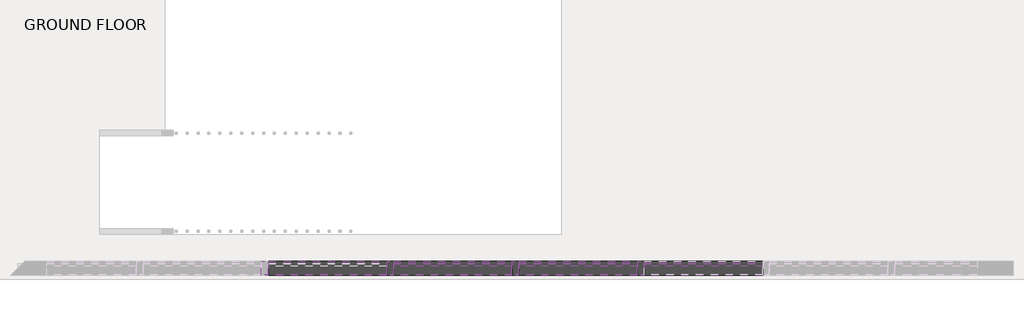
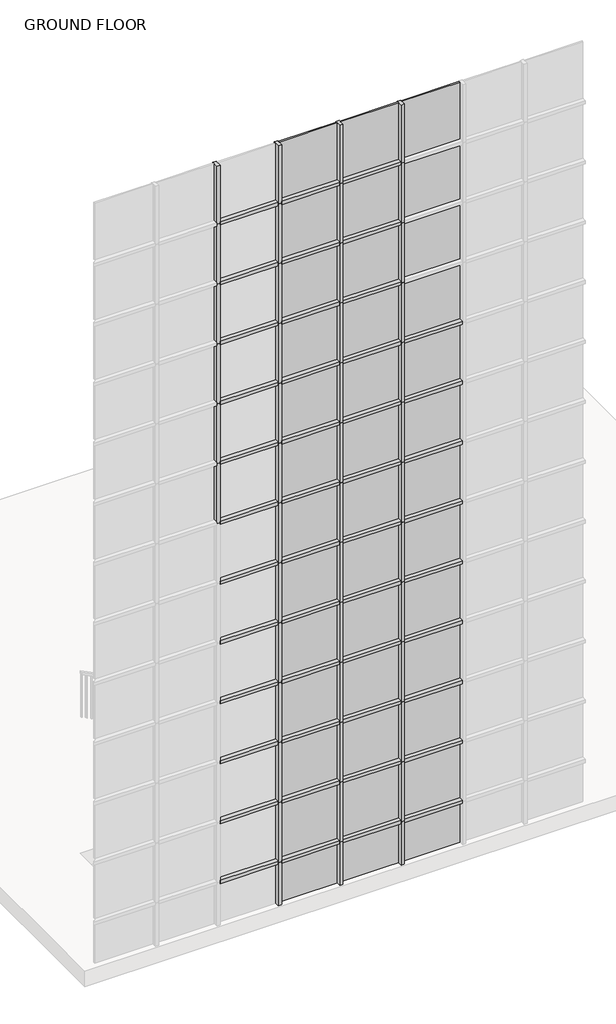
# One storey, part 3 of 16: 90 members, 39 plates.
"""IFC4 building model written with IfcOpenShell, lengths in millimetres."""

from ifc_helpers import new_model, si_unit, origin, place, context, project, spatial, transform, mapped, element, save
from components import member_d518c94e, member_b860638c, member_31fee25f, system_panel_glazed_5cba32e5

model = new_model("IFC4")

# Units and contexts
model_context = context("Model", 3, world=origin())
ifc_project = project(units=[si_unit("LENGTHUNIT", "METRE", prefix="MILLI")], contexts=[model_context])

# Site, building, storey
site = spatial("IfcSite", under=ifc_project)
building = spatial("IfcBuilding", under=site)
storey = spatial("IfcBuildingStorey", under=building, Name="GROUND FLOOR", Elevation=0.0)

# Members
placement = place(None, origin())
member_shape = member_d518c94e(model_context)
element("IfcMember", 1, ObjectType="Rectangular Mullion : 2.5\" x 5\" rectangular", at=placement, inside=storey, context=model_context, shape_type="MappedRepresentation", body=[
    mapped(member_shape, transform((-5691.994061, -5739.2238032, 1168.8884615), x_axis=(0.0, 0.0, 1.0), y_axis=(0.0, -1.0, 0.0), z_axis=(1.0, 0.0, 0.0))),
])
element("IfcMember", 2, ObjectType="Rectangular Mullion : 2.5\" x 5\" rectangular", at=placement, inside=storey, context=model_context, shape_type="MappedRepresentation", body=[
    mapped(member_shape, transform((-4526.5248302, -5739.2238032, 1168.8884615), x_axis=(0.0, 0.0, 1.0), y_axis=(0.0, -1.0, 0.0), z_axis=(1.0, 0.0, 0.0))),
])
element("IfcMember", 3, ObjectType="Rectangular Mullion : 2.5\" x 5\" rectangular", at=placement, inside=storey, context=model_context, shape_type="MappedRepresentation", body=[
    mapped(member_shape, transform((-3361.0555995, -5739.2238032, 1168.8884615), x_axis=(0.0, 0.0, 1.0), y_axis=(0.0, -1.0, 0.0), z_axis=(1.0, 0.0, 0.0))),
])
element("IfcMember", 4, ObjectType="Rectangular Mullion : 2.5\" x 5\" rectangular", at=placement, inside=storey, context=model_context, shape_type="MappedRepresentation", body=[
    mapped(member_shape, transform((-2195.5863688, -5739.2238032, 1168.8884615), x_axis=(0.0, 0.0, 1.0), y_axis=(0.0, -1.0, 0.0), z_axis=(1.0, 0.0, 0.0))),
])
element("IfcMember", 5, ObjectType="Rectangular Mullion : 2.5\" x 5\" rectangular", at=placement, inside=storey, context=model_context, shape_type="MappedRepresentation", body=[
    mapped(member_shape, transform((-5691.994061, -5739.2238032, 2369.5269231), x_axis=(0.0, 0.0, 1.0), y_axis=(0.0, -1.0, 0.0), z_axis=(1.0, 0.0, 0.0))),
])
element("IfcMember", 6, ObjectType="Rectangular Mullion : 2.5\" x 5\" rectangular", at=placement, inside=storey, context=model_context, shape_type="MappedRepresentation", body=[
    mapped(member_shape, transform((-4526.5248302, -5739.2238032, 2369.5269231), x_axis=(0.0, 0.0, 1.0), y_axis=(0.0, -1.0, 0.0), z_axis=(1.0, 0.0, 0.0))),
])
element("IfcMember", 7, ObjectType="Rectangular Mullion : 2.5\" x 5\" rectangular", at=placement, inside=storey, context=model_context, shape_type="MappedRepresentation", body=[
    mapped(member_shape, transform((-3361.0555995, -5739.2238032, 2369.5269231), x_axis=(0.0, 0.0, 1.0), y_axis=(0.0, -1.0, 0.0), z_axis=(1.0, 0.0, 0.0))),
])
element("IfcMember", 8, ObjectType="Rectangular Mullion : 2.5\" x 5\" rectangular", at=placement, inside=storey, context=model_context, shape_type="MappedRepresentation", body=[
    mapped(member_shape, transform((-2195.5863688, -5739.2238032, 2369.5269231), x_axis=(0.0, 0.0, 1.0), y_axis=(0.0, -1.0, 0.0), z_axis=(1.0, 0.0, 0.0))),
])
element("IfcMember", 9, ObjectType="Rectangular Mullion : 2.5\" x 5\" rectangular", at=placement, inside=storey, context=model_context, shape_type="MappedRepresentation", body=[
    mapped(member_shape, transform((-5691.994061, -5739.2238032, 3570.1653846), x_axis=(0.0, 0.0, 1.0), y_axis=(0.0, -1.0, 0.0), z_axis=(1.0, 0.0, 0.0))),
])
element("IfcMember", 10, ObjectType="Rectangular Mullion : 2.5\" x 5\" rectangular", at=placement, inside=storey, context=model_context, shape_type="MappedRepresentation", body=[
    mapped(member_shape, transform((-4526.5248302, -5739.2238032, 3570.1653846), x_axis=(0.0, 0.0, 1.0), y_axis=(0.0, -1.0, 0.0), z_axis=(1.0, 0.0, 0.0))),
])
element("IfcMember", 11, ObjectType="Rectangular Mullion : 2.5\" x 5\" rectangular", at=placement, inside=storey, context=model_context, shape_type="MappedRepresentation", body=[
    mapped(member_shape, transform((-3361.0555995, -5739.2238032, 3570.1653846), x_axis=(0.0, 0.0, 1.0), y_axis=(0.0, -1.0, 0.0), z_axis=(1.0, 0.0, 0.0))),
])
element("IfcMember", 12, ObjectType="Rectangular Mullion : 2.5\" x 5\" rectangular", at=placement, inside=storey, context=model_context, shape_type="MappedRepresentation", body=[
    mapped(member_shape, transform((-2195.5863688, -5739.2238032, 3570.1653846), x_axis=(0.0, 0.0, 1.0), y_axis=(0.0, -1.0, 0.0), z_axis=(1.0, 0.0, 0.0))),
])
element("IfcMember", 13, ObjectType="Rectangular Mullion : 2.5\" x 5\" rectangular", at=placement, inside=storey, context=model_context, shape_type="MappedRepresentation", body=[
    mapped(member_shape, transform((-5691.994061, -5739.2238032, 4770.8038462), x_axis=(0.0, 0.0, 1.0), y_axis=(0.0, -1.0, 0.0), z_axis=(1.0, 0.0, 0.0))),
])
element("IfcMember", 14, ObjectType="Rectangular Mullion : 2.5\" x 5\" rectangular", at=placement, inside=storey, context=model_context, shape_type="MappedRepresentation", body=[
    mapped(member_shape, transform((-4526.5248302, -5739.2238032, 4770.8038462), x_axis=(0.0, 0.0, 1.0), y_axis=(0.0, -1.0, 0.0), z_axis=(1.0, 0.0, 0.0))),
])
element("IfcMember", 15, ObjectType="Rectangular Mullion : 2.5\" x 5\" rectangular", at=placement, inside=storey, context=model_context, shape_type="MappedRepresentation", body=[
    mapped(member_shape, transform((-3361.0555995, -5739.2238032, 4770.8038462), x_axis=(0.0, 0.0, 1.0), y_axis=(0.0, -1.0, 0.0), z_axis=(1.0, 0.0, 0.0))),
])
element("IfcMember", 16, ObjectType="Rectangular Mullion : 2.5\" x 5\" rectangular", at=placement, inside=storey, context=model_context, shape_type="MappedRepresentation", body=[
    mapped(member_shape, transform((-2195.5863688, -5739.2238032, 4770.8038462), x_axis=(0.0, 0.0, 1.0), y_axis=(0.0, -1.0, 0.0), z_axis=(1.0, 0.0, 0.0))),
])
element("IfcMember", 17, ObjectType="Rectangular Mullion : 2.5\" x 5\" rectangular", at=placement, inside=storey, context=model_context, shape_type="MappedRepresentation", body=[
    mapped(member_shape, transform((-5691.994061, -5739.2238032, 5971.4423077), x_axis=(0.0, 0.0, 1.0), y_axis=(0.0, -1.0, 0.0), z_axis=(1.0, 0.0, 0.0))),
])
element("IfcMember", 18, ObjectType="Rectangular Mullion : 2.5\" x 5\" rectangular", at=placement, inside=storey, context=model_context, shape_type="MappedRepresentation", body=[
    mapped(member_shape, transform((-4526.5248302, -5739.2238032, 5971.4423077), x_axis=(0.0, 0.0, 1.0), y_axis=(0.0, -1.0, 0.0), z_axis=(1.0, 0.0, 0.0))),
])
element("IfcMember", 19, ObjectType="Rectangular Mullion : 2.5\" x 5\" rectangular", at=placement, inside=storey, context=model_context, shape_type="MappedRepresentation", body=[
    mapped(member_shape, transform((-3361.0555995, -5739.2238032, 5971.4423077), x_axis=(0.0, 0.0, 1.0), y_axis=(0.0, -1.0, 0.0), z_axis=(1.0, 0.0, 0.0))),
])
element("IfcMember", 20, ObjectType="Rectangular Mullion : 2.5\" x 5\" rectangular", at=placement, inside=storey, context=model_context, shape_type="MappedRepresentation", body=[
    mapped(member_shape, transform((-2195.5863688, -5739.2238032, 5971.4423077), x_axis=(0.0, 0.0, 1.0), y_axis=(0.0, -1.0, 0.0), z_axis=(1.0, 0.0, 0.0))),
])
element("IfcMember", 21, ObjectType="Rectangular Mullion : 2.5\" x 5\" rectangular", at=placement, inside=storey, context=model_context, shape_type="MappedRepresentation", body=[
    mapped(member_shape, transform((-5691.994061, -5739.2238032, 7172.0807692), x_axis=(0.0, 0.0, 1.0), y_axis=(0.0, -1.0, 0.0), z_axis=(1.0, 0.0, 0.0))),
])
element("IfcMember", 22, ObjectType="Rectangular Mullion : 2.5\" x 5\" rectangular", at=placement, inside=storey, context=model_context, shape_type="MappedRepresentation", body=[
    mapped(member_shape, transform((-4526.5248302, -5739.2238032, 7172.0807692), x_axis=(0.0, 0.0, 1.0), y_axis=(0.0, -1.0, 0.0), z_axis=(1.0, 0.0, 0.0))),
])
element("IfcMember", 23, ObjectType="Rectangular Mullion : 2.5\" x 5\" rectangular", at=placement, inside=storey, context=model_context, shape_type="MappedRepresentation", body=[
    mapped(member_shape, transform((-3361.0555995, -5739.2238032, 7172.0807692), x_axis=(0.0, 0.0, 1.0), y_axis=(0.0, -1.0, 0.0), z_axis=(1.0, 0.0, 0.0))),
])
element("IfcMember", 24, ObjectType="Rectangular Mullion : 2.5\" x 5\" rectangular", at=placement, inside=storey, context=model_context, shape_type="MappedRepresentation", body=[
    mapped(member_shape, transform((-2195.5863688, -5739.2238032, 7172.0807692), x_axis=(0.0, 0.0, 1.0), y_axis=(0.0, -1.0, 0.0), z_axis=(1.0, 0.0, 0.0))),
])
element("IfcMember", 25, ObjectType="Rectangular Mullion : 2.5\" x 5\" rectangular", at=placement, inside=storey, context=model_context, shape_type="MappedRepresentation", body=[
    mapped(member_shape, transform((-5691.994061, -5739.2238032, 8372.7192308), x_axis=(0.0, 0.0, 1.0), y_axis=(0.0, -1.0, 0.0), z_axis=(1.0, 0.0, 0.0))),
])
element("IfcMember", 26, ObjectType="Rectangular Mullion : 2.5\" x 5\" rectangular", at=placement, inside=storey, context=model_context, shape_type="MappedRepresentation", body=[
    mapped(member_shape, transform((-4526.5248302, -5739.2238032, 8372.7192308), x_axis=(0.0, 0.0, 1.0), y_axis=(0.0, -1.0, 0.0), z_axis=(1.0, 0.0, 0.0))),
])
element("IfcMember", 27, ObjectType="Rectangular Mullion : 2.5\" x 5\" rectangular", at=placement, inside=storey, context=model_context, shape_type="MappedRepresentation", body=[
    mapped(member_shape, transform((-3361.0555995, -5739.2238032, 8372.7192308), x_axis=(0.0, 0.0, 1.0), y_axis=(0.0, -1.0, 0.0), z_axis=(1.0, 0.0, 0.0))),
])
element("IfcMember", 28, ObjectType="Rectangular Mullion : 2.5\" x 5\" rectangular", at=placement, inside=storey, context=model_context, shape_type="MappedRepresentation", body=[
    mapped(member_shape, transform((-2195.5863688, -5739.2238032, 8372.7192308), x_axis=(0.0, 0.0, 1.0), y_axis=(0.0, -1.0, 0.0), z_axis=(1.0, 0.0, 0.0))),
])
element("IfcMember", 29, ObjectType="Rectangular Mullion : 2.5\" x 5\" rectangular", at=placement, inside=storey, context=model_context, shape_type="MappedRepresentation", body=[
    mapped(member_shape, transform((-5691.994061, -5739.2238032, 9573.3576923), x_axis=(0.0, 0.0, 1.0), y_axis=(0.0, -1.0, 0.0), z_axis=(1.0, 0.0, 0.0))),
])
element("IfcMember", 30, ObjectType="Rectangular Mullion : 2.5\" x 5\" rectangular", at=placement, inside=storey, context=model_context, shape_type="MappedRepresentation", body=[
    mapped(member_shape, transform((-4526.5248302, -5739.2238032, 9573.3576923), x_axis=(0.0, 0.0, 1.0), y_axis=(0.0, -1.0, 0.0), z_axis=(1.0, 0.0, 0.0))),
])
element("IfcMember", 31, ObjectType="Rectangular Mullion : 2.5\" x 5\" rectangular", at=placement, inside=storey, context=model_context, shape_type="MappedRepresentation", body=[
    mapped(member_shape, transform((-3361.0555995, -5739.2238032, 9573.3576923), x_axis=(0.0, 0.0, 1.0), y_axis=(0.0, -1.0, 0.0), z_axis=(1.0, 0.0, 0.0))),
])
element("IfcMember", 32, ObjectType="Rectangular Mullion : 2.5\" x 5\" rectangular", at=placement, inside=storey, context=model_context, shape_type="MappedRepresentation", body=[
    mapped(member_shape, transform((-2195.5863688, -5739.2238032, 9573.3576923), x_axis=(0.0, 0.0, 1.0), y_axis=(0.0, -1.0, 0.0), z_axis=(1.0, 0.0, 0.0))),
])
element("IfcMember", 33, ObjectType="Rectangular Mullion : 2.5\" x 5\" rectangular", at=placement, inside=storey, context=model_context, shape_type="MappedRepresentation", body=[
    mapped(member_shape, transform((-5691.994061, -5739.2238032, 10773.9961538), x_axis=(0.0, 0.0, 1.0), y_axis=(0.0, -1.0, 0.0), z_axis=(1.0, 0.0, 0.0))),
])
element("IfcMember", 34, ObjectType="Rectangular Mullion : 2.5\" x 5\" rectangular", at=placement, inside=storey, context=model_context, shape_type="MappedRepresentation", body=[
    mapped(member_shape, transform((-4526.5248302, -5739.2238032, 10773.9961538), x_axis=(0.0, 0.0, 1.0), y_axis=(0.0, -1.0, 0.0), z_axis=(1.0, 0.0, 0.0))),
])
element("IfcMember", 35, ObjectType="Rectangular Mullion : 2.5\" x 5\" rectangular", at=placement, inside=storey, context=model_context, shape_type="MappedRepresentation", body=[
    mapped(member_shape, transform((-3361.0555995, -5739.2238032, 10773.9961538), x_axis=(0.0, 0.0, 1.0), y_axis=(0.0, -1.0, 0.0), z_axis=(1.0, 0.0, 0.0))),
])
element("IfcMember", 36, ObjectType="Rectangular Mullion : 2.5\" x 5\" rectangular", at=placement, inside=storey, context=model_context, shape_type="MappedRepresentation", body=[
    mapped(member_shape, transform((-2195.5863688, -5739.2238032, 10773.9961538), x_axis=(0.0, 0.0, 1.0), y_axis=(0.0, -1.0, 0.0), z_axis=(1.0, 0.0, 0.0))),
])
element("IfcMember", 37, ObjectType="Rectangular Mullion : 2.5\" x 5\" rectangular", at=placement, inside=storey, context=model_context, shape_type="MappedRepresentation", body=[
    mapped(member_shape, transform((-5691.994061, -5739.2238032, 11974.6346154), x_axis=(0.0, 0.0, 1.0), y_axis=(0.0, -1.0, 0.0), z_axis=(1.0, 0.0, 0.0))),
])
element("IfcMember", 38, ObjectType="Rectangular Mullion : 2.5\" x 5\" rectangular", at=placement, inside=storey, context=model_context, shape_type="MappedRepresentation", body=[
    mapped(member_shape, transform((-4526.5248302, -5739.2238032, 11974.6346154), x_axis=(0.0, 0.0, 1.0), y_axis=(0.0, -1.0, 0.0), z_axis=(1.0, 0.0, 0.0))),
])
element("IfcMember", 39, ObjectType="Rectangular Mullion : 2.5\" x 5\" rectangular", at=placement, inside=storey, context=model_context, shape_type="MappedRepresentation", body=[
    mapped(member_shape, transform((-3361.0555995, -5739.2238032, 11974.6346154), x_axis=(0.0, 0.0, 1.0), y_axis=(0.0, -1.0, 0.0), z_axis=(1.0, 0.0, 0.0))),
])
element("IfcMember", 40, ObjectType="Rectangular Mullion : 2.5\" x 5\" rectangular", at=placement, inside=storey, context=model_context, shape_type="MappedRepresentation", body=[
    mapped(member_shape, transform((-5691.994061, -5739.2238032, 13175.2730769), x_axis=(0.0, 0.0, 1.0), y_axis=(0.0, -1.0, 0.0), z_axis=(1.0, 0.0, 0.0))),
])
element("IfcMember", 41, ObjectType="Rectangular Mullion : 2.5\" x 5\" rectangular", at=placement, inside=storey, context=model_context, shape_type="MappedRepresentation", body=[
    mapped(member_shape, transform((-4526.5248302, -5739.2238032, 13175.2730769), x_axis=(0.0, 0.0, 1.0), y_axis=(0.0, -1.0, 0.0), z_axis=(1.0, 0.0, 0.0))),
])
element("IfcMember", 42, ObjectType="Rectangular Mullion : 2.5\" x 5\" rectangular", at=placement, inside=storey, context=model_context, shape_type="MappedRepresentation", body=[
    mapped(member_shape, transform((-3361.0555995, -5739.2238032, 13175.2730769), x_axis=(0.0, 0.0, 1.0), y_axis=(0.0, -1.0, 0.0), z_axis=(1.0, 0.0, 0.0))),
])
element("IfcMember", 43, ObjectType="Rectangular Mullion : 2.5\" x 5\" rectangular", at=placement, inside=storey, context=model_context, shape_type="MappedRepresentation", body=[
    mapped(member_shape, transform((-5691.994061, -5739.2238032, 14375.9115385), x_axis=(0.0, 0.0, 1.0), y_axis=(0.0, -1.0, 0.0), z_axis=(1.0, 0.0, 0.0))),
])
element("IfcMember", 44, ObjectType="Rectangular Mullion : 2.5\" x 5\" rectangular", at=placement, inside=storey, context=model_context, shape_type="MappedRepresentation", body=[
    mapped(member_shape, transform((-4526.5248302, -5739.2238032, 14375.9115385), x_axis=(0.0, 0.0, 1.0), y_axis=(0.0, -1.0, 0.0), z_axis=(1.0, 0.0, 0.0))),
])
element("IfcMember", 45, ObjectType="Rectangular Mullion : 2.5\" x 5\" rectangular", at=placement, inside=storey, context=model_context, shape_type="MappedRepresentation", body=[
    mapped(member_shape, transform((-3361.0555995, -5739.2238032, 14375.9115385), x_axis=(0.0, 0.0, 1.0), y_axis=(0.0, -1.0, 0.0), z_axis=(1.0, 0.0, 0.0))),
])
member_2_shape = member_b860638c(model_context)
element("IfcMember", 46, ObjectType="Rectangular Mullion : 2.5\" x 5\" rectangular", at=placement, inside=storey, context=model_context, shape_type="MappedRepresentation", body=[
    mapped(member_2_shape, transform((-5660.244061, -5739.2238032, 0.0), x_axis=(1.0, 0.0, 0.0), y_axis=(0.0, -1.0, 0.0), z_axis=(0.0, 0.0, -1.0))),
])
element("IfcMember", 47, ObjectType="Rectangular Mullion : 2.5\" x 5\" rectangular", at=placement, inside=storey, context=model_context, shape_type="MappedRepresentation", body=[
    mapped(member_2_shape, transform((-4494.7748302, -5739.2238032, 0.0), x_axis=(1.0, 0.0, 0.0), y_axis=(0.0, -1.0, 0.0), z_axis=(0.0, 0.0, -1.0))),
])
element("IfcMember", 48, ObjectType="Rectangular Mullion : 2.5\" x 5\" rectangular", at=placement, inside=storey, context=model_context, shape_type="MappedRepresentation", body=[
    mapped(member_2_shape, transform((-3329.3055995, -5739.2238032, 0.0), x_axis=(1.0, 0.0, 0.0), y_axis=(0.0, -1.0, 0.0), z_axis=(0.0, 0.0, -1.0))),
])
member_3_shape = member_31fee25f(model_context)
element("IfcMember", 49, ObjectType="Rectangular Mullion : 2.5\" x 5\" rectangular", at=placement, inside=storey, context=model_context, shape_type="MappedRepresentation", body=[
    mapped(member_3_shape, transform((-5660.244061, -5739.2238032, 1168.8884615), x_axis=(1.0, 0.0, 0.0), y_axis=(0.0, -1.0, 0.0), z_axis=(0.0, 0.0, -1.0))),
])
element("IfcMember", 50, ObjectType="Rectangular Mullion : 2.5\" x 5\" rectangular", at=placement, inside=storey, context=model_context, shape_type="MappedRepresentation", body=[
    mapped(member_3_shape, transform((-4494.7748302, -5739.2238032, 1168.8884615), x_axis=(1.0, 0.0, 0.0), y_axis=(0.0, -1.0, 0.0), z_axis=(0.0, 0.0, -1.0))),
])
element("IfcMember", 51, ObjectType="Rectangular Mullion : 2.5\" x 5\" rectangular", at=placement, inside=storey, context=model_context, shape_type="MappedRepresentation", body=[
    mapped(member_3_shape, transform((-3329.3055995, -5739.2238032, 1168.8884615), x_axis=(1.0, 0.0, 0.0), y_axis=(0.0, -1.0, 0.0), z_axis=(0.0, 0.0, -1.0))),
])
element("IfcMember", 52, ObjectType="Rectangular Mullion : 2.5\" x 5\" rectangular", at=placement, inside=storey, context=model_context, shape_type="MappedRepresentation", body=[
    mapped(member_3_shape, transform((-5660.244061, -5739.2238032, 2369.5269231), x_axis=(1.0, 0.0, 0.0), y_axis=(0.0, -1.0, 0.0), z_axis=(0.0, 0.0, -1.0))),
])
element("IfcMember", 53, ObjectType="Rectangular Mullion : 2.5\" x 5\" rectangular", at=placement, inside=storey, context=model_context, shape_type="MappedRepresentation", body=[
    mapped(member_3_shape, transform((-4494.7748302, -5739.2238032, 2369.5269231), x_axis=(1.0, 0.0, 0.0), y_axis=(0.0, -1.0, 0.0), z_axis=(0.0, 0.0, -1.0))),
])
element("IfcMember", 54, ObjectType="Rectangular Mullion : 2.5\" x 5\" rectangular", at=placement, inside=storey, context=model_context, shape_type="MappedRepresentation", body=[
    mapped(member_3_shape, transform((-3329.3055995, -5739.2238032, 2369.5269231), x_axis=(1.0, 0.0, 0.0), y_axis=(0.0, -1.0, 0.0), z_axis=(0.0, 0.0, -1.0))),
])
element("IfcMember", 55, ObjectType="Rectangular Mullion : 2.5\" x 5\" rectangular", at=placement, inside=storey, context=model_context, shape_type="MappedRepresentation", body=[
    mapped(member_3_shape, transform((-5660.244061, -5739.2238032, 3570.1653846), x_axis=(1.0, 0.0, 0.0), y_axis=(0.0, -1.0, 0.0), z_axis=(0.0, 0.0, -1.0))),
])
element("IfcMember", 56, ObjectType="Rectangular Mullion : 2.5\" x 5\" rectangular", at=placement, inside=storey, context=model_context, shape_type="MappedRepresentation", body=[
    mapped(member_3_shape, transform((-4494.7748302, -5739.2238032, 3570.1653846), x_axis=(1.0, 0.0, 0.0), y_axis=(0.0, -1.0, 0.0), z_axis=(0.0, 0.0, -1.0))),
])
element("IfcMember", 57, ObjectType="Rectangular Mullion : 2.5\" x 5\" rectangular", at=placement, inside=storey, context=model_context, shape_type="MappedRepresentation", body=[
    mapped(member_3_shape, transform((-3329.3055995, -5739.2238032, 3570.1653846), x_axis=(1.0, 0.0, 0.0), y_axis=(0.0, -1.0, 0.0), z_axis=(0.0, 0.0, -1.0))),
])
element("IfcMember", 58, ObjectType="Rectangular Mullion : 2.5\" x 5\" rectangular", at=placement, inside=storey, context=model_context, shape_type="MappedRepresentation", body=[
    mapped(member_3_shape, transform((-5660.244061, -5739.2238032, 4770.8038462), x_axis=(1.0, 0.0, 0.0), y_axis=(0.0, -1.0, 0.0), z_axis=(0.0, 0.0, -1.0))),
])
element("IfcMember", 59, ObjectType="Rectangular Mullion : 2.5\" x 5\" rectangular", at=placement, inside=storey, context=model_context, shape_type="MappedRepresentation", body=[
    mapped(member_3_shape, transform((-4494.7748302, -5739.2238032, 4770.8038462), x_axis=(1.0, 0.0, 0.0), y_axis=(0.0, -1.0, 0.0), z_axis=(0.0, 0.0, -1.0))),
])
element("IfcMember", 60, ObjectType="Rectangular Mullion : 2.5\" x 5\" rectangular", at=placement, inside=storey, context=model_context, shape_type="MappedRepresentation", body=[
    mapped(member_3_shape, transform((-3329.3055995, -5739.2238032, 4770.8038462), x_axis=(1.0, 0.0, 0.0), y_axis=(0.0, -1.0, 0.0), z_axis=(0.0, 0.0, -1.0))),
])
element("IfcMember", 61, ObjectType="Rectangular Mullion : 2.5\" x 5\" rectangular", at=placement, inside=storey, context=model_context, shape_type="MappedRepresentation", body=[
    mapped(member_3_shape, transform((-5660.244061, -5739.2238032, 5971.4423077), x_axis=(1.0, 0.0, 0.0), y_axis=(0.0, -1.0, 0.0), z_axis=(0.0, 0.0, -1.0))),
])
element("IfcMember", 62, ObjectType="Rectangular Mullion : 2.5\" x 5\" rectangular", at=placement, inside=storey, context=model_context, shape_type="MappedRepresentation", body=[
    mapped(member_3_shape, transform((-4494.7748302, -5739.2238032, 5971.4423077), x_axis=(1.0, 0.0, 0.0), y_axis=(0.0, -1.0, 0.0), z_axis=(0.0, 0.0, -1.0))),
])
element("IfcMember", 63, ObjectType="Rectangular Mullion : 2.5\" x 5\" rectangular", at=placement, inside=storey, context=model_context, shape_type="MappedRepresentation", body=[
    mapped(member_3_shape, transform((-3329.3055995, -5739.2238032, 5971.4423077), x_axis=(1.0, 0.0, 0.0), y_axis=(0.0, -1.0, 0.0), z_axis=(0.0, 0.0, -1.0))),
])
element("IfcMember", 64, ObjectType="Rectangular Mullion : 2.5\" x 5\" rectangular", at=placement, inside=storey, context=model_context, shape_type="MappedRepresentation", body=[
    mapped(member_3_shape, transform((-5660.244061, -5739.2238032, 7172.0807692), x_axis=(1.0, 0.0, 0.0), y_axis=(0.0, -1.0, 0.0), z_axis=(0.0, 0.0, -1.0))),
])
element("IfcMember", 65, ObjectType="Rectangular Mullion : 2.5\" x 5\" rectangular", at=placement, inside=storey, context=model_context, shape_type="MappedRepresentation", body=[
    mapped(member_3_shape, transform((-4494.7748302, -5739.2238032, 7172.0807692), x_axis=(1.0, 0.0, 0.0), y_axis=(0.0, -1.0, 0.0), z_axis=(0.0, 0.0, -1.0))),
])
element("IfcMember", 66, ObjectType="Rectangular Mullion : 2.5\" x 5\" rectangular", at=placement, inside=storey, context=model_context, shape_type="MappedRepresentation", body=[
    mapped(member_3_shape, transform((-3329.3055995, -5739.2238032, 7172.0807692), x_axis=(1.0, 0.0, 0.0), y_axis=(0.0, -1.0, 0.0), z_axis=(0.0, 0.0, -1.0))),
])
element("IfcMember", 67, ObjectType="Rectangular Mullion : 2.5\" x 5\" rectangular", at=placement, inside=storey, context=model_context, shape_type="MappedRepresentation", body=[
    mapped(member_3_shape, transform((-6825.7132917, -5739.2238032, 8372.7192308), x_axis=(1.0, 0.0, 0.0), y_axis=(0.0, -1.0, 0.0), z_axis=(0.0, 0.0, -1.0))),
])
element("IfcMember", 68, ObjectType="Rectangular Mullion : 2.5\" x 5\" rectangular", at=placement, inside=storey, context=model_context, shape_type="MappedRepresentation", body=[
    mapped(member_3_shape, transform((-5660.244061, -5739.2238032, 8372.7192308), x_axis=(1.0, 0.0, 0.0), y_axis=(0.0, -1.0, 0.0), z_axis=(0.0, 0.0, -1.0))),
])
element("IfcMember", 69, ObjectType="Rectangular Mullion : 2.5\" x 5\" rectangular", at=placement, inside=storey, context=model_context, shape_type="MappedRepresentation", body=[
    mapped(member_3_shape, transform((-4494.7748302, -5739.2238032, 8372.7192308), x_axis=(1.0, 0.0, 0.0), y_axis=(0.0, -1.0, 0.0), z_axis=(0.0, 0.0, -1.0))),
])
element("IfcMember", 70, ObjectType="Rectangular Mullion : 2.5\" x 5\" rectangular", at=placement, inside=storey, context=model_context, shape_type="MappedRepresentation", body=[
    mapped(member_3_shape, transform((-3329.3055995, -5739.2238032, 8372.7192308), x_axis=(1.0, 0.0, 0.0), y_axis=(0.0, -1.0, 0.0), z_axis=(0.0, 0.0, -1.0))),
])
element("IfcMember", 71, ObjectType="Rectangular Mullion : 2.5\" x 5\" rectangular", at=placement, inside=storey, context=model_context, shape_type="MappedRepresentation", body=[
    mapped(member_3_shape, transform((-6825.7132917, -5739.2238032, 9573.3576923), x_axis=(1.0, 0.0, 0.0), y_axis=(0.0, -1.0, 0.0), z_axis=(0.0, 0.0, -1.0))),
])
element("IfcMember", 72, ObjectType="Rectangular Mullion : 2.5\" x 5\" rectangular", at=placement, inside=storey, context=model_context, shape_type="MappedRepresentation", body=[
    mapped(member_3_shape, transform((-5660.244061, -5739.2238032, 9573.3576923), x_axis=(1.0, 0.0, 0.0), y_axis=(0.0, -1.0, 0.0), z_axis=(0.0, 0.0, -1.0))),
])
element("IfcMember", 73, ObjectType="Rectangular Mullion : 2.5\" x 5\" rectangular", at=placement, inside=storey, context=model_context, shape_type="MappedRepresentation", body=[
    mapped(member_3_shape, transform((-4494.7748302, -5739.2238032, 9573.3576923), x_axis=(1.0, 0.0, 0.0), y_axis=(0.0, -1.0, 0.0), z_axis=(0.0, 0.0, -1.0))),
])
element("IfcMember", 74, ObjectType="Rectangular Mullion : 2.5\" x 5\" rectangular", at=placement, inside=storey, context=model_context, shape_type="MappedRepresentation", body=[
    mapped(member_3_shape, transform((-3329.3055995, -5739.2238032, 9573.3576923), x_axis=(1.0, 0.0, 0.0), y_axis=(0.0, -1.0, 0.0), z_axis=(0.0, 0.0, -1.0))),
])
element("IfcMember", 75, ObjectType="Rectangular Mullion : 2.5\" x 5\" rectangular", at=placement, inside=storey, context=model_context, shape_type="MappedRepresentation", body=[
    mapped(member_3_shape, transform((-6825.7132917, -5739.2238032, 10773.9961538), x_axis=(1.0, 0.0, 0.0), y_axis=(0.0, -1.0, 0.0), z_axis=(0.0, 0.0, -1.0))),
])
element("IfcMember", 76, ObjectType="Rectangular Mullion : 2.5\" x 5\" rectangular", at=placement, inside=storey, context=model_context, shape_type="MappedRepresentation", body=[
    mapped(member_3_shape, transform((-5660.244061, -5739.2238032, 10773.9961538), x_axis=(1.0, 0.0, 0.0), y_axis=(0.0, -1.0, 0.0), z_axis=(0.0, 0.0, -1.0))),
])
element("IfcMember", 77, ObjectType="Rectangular Mullion : 2.5\" x 5\" rectangular", at=placement, inside=storey, context=model_context, shape_type="MappedRepresentation", body=[
    mapped(member_3_shape, transform((-4494.7748302, -5739.2238032, 10773.9961538), x_axis=(1.0, 0.0, 0.0), y_axis=(0.0, -1.0, 0.0), z_axis=(0.0, 0.0, -1.0))),
])
element("IfcMember", 78, ObjectType="Rectangular Mullion : 2.5\" x 5\" rectangular", at=placement, inside=storey, context=model_context, shape_type="MappedRepresentation", body=[
    mapped(member_3_shape, transform((-3329.3055995, -5739.2238032, 10773.9961538), x_axis=(1.0, 0.0, 0.0), y_axis=(0.0, -1.0, 0.0), z_axis=(0.0, 0.0, -1.0))),
])
element("IfcMember", 79, ObjectType="Rectangular Mullion : 2.5\" x 5\" rectangular", at=placement, inside=storey, context=model_context, shape_type="MappedRepresentation", body=[
    mapped(member_3_shape, transform((-6825.7132917, -5739.2238032, 11974.6346154), x_axis=(1.0, 0.0, 0.0), y_axis=(0.0, -1.0, 0.0), z_axis=(0.0, 0.0, -1.0))),
])
element("IfcMember", 80, ObjectType="Rectangular Mullion : 2.5\" x 5\" rectangular", at=placement, inside=storey, context=model_context, shape_type="MappedRepresentation", body=[
    mapped(member_3_shape, transform((-5660.244061, -5739.2238032, 11974.6346154), x_axis=(1.0, 0.0, 0.0), y_axis=(0.0, -1.0, 0.0), z_axis=(0.0, 0.0, -1.0))),
])
element("IfcMember", 81, ObjectType="Rectangular Mullion : 2.5\" x 5\" rectangular", at=placement, inside=storey, context=model_context, shape_type="MappedRepresentation", body=[
    mapped(member_3_shape, transform((-4494.7748302, -5739.2238032, 11974.6346154), x_axis=(1.0, 0.0, 0.0), y_axis=(0.0, -1.0, 0.0), z_axis=(0.0, 0.0, -1.0))),
])
element("IfcMember", 82, ObjectType="Rectangular Mullion : 2.5\" x 5\" rectangular", at=placement, inside=storey, context=model_context, shape_type="MappedRepresentation", body=[
    mapped(member_3_shape, transform((-3329.3055995, -5739.2238032, 11974.6346154), x_axis=(1.0, 0.0, 0.0), y_axis=(0.0, -1.0, 0.0), z_axis=(0.0, 0.0, -1.0))),
])
element("IfcMember", 83, ObjectType="Rectangular Mullion : 2.5\" x 5\" rectangular", at=placement, inside=storey, context=model_context, shape_type="MappedRepresentation", body=[
    mapped(member_3_shape, transform((-6825.7132917, -5739.2238032, 13175.2730769), x_axis=(1.0, 0.0, 0.0), y_axis=(0.0, -1.0, 0.0), z_axis=(0.0, 0.0, -1.0))),
])
element("IfcMember", 84, ObjectType="Rectangular Mullion : 2.5\" x 5\" rectangular", at=placement, inside=storey, context=model_context, shape_type="MappedRepresentation", body=[
    mapped(member_3_shape, transform((-5660.244061, -5739.2238032, 13175.2730769), x_axis=(1.0, 0.0, 0.0), y_axis=(0.0, -1.0, 0.0), z_axis=(0.0, 0.0, -1.0))),
])
element("IfcMember", 85, ObjectType="Rectangular Mullion : 2.5\" x 5\" rectangular", at=placement, inside=storey, context=model_context, shape_type="MappedRepresentation", body=[
    mapped(member_3_shape, transform((-4494.7748302, -5739.2238032, 13175.2730769), x_axis=(1.0, 0.0, 0.0), y_axis=(0.0, -1.0, 0.0), z_axis=(0.0, 0.0, -1.0))),
])
element("IfcMember", 86, ObjectType="Rectangular Mullion : 2.5\" x 5\" rectangular", at=placement, inside=storey, context=model_context, shape_type="MappedRepresentation", body=[
    mapped(member_3_shape, transform((-3329.3055995, -5739.2238032, 13175.2730769), x_axis=(1.0, 0.0, 0.0), y_axis=(0.0, -1.0, 0.0), z_axis=(0.0, 0.0, -1.0))),
])
element("IfcMember", 87, ObjectType="Rectangular Mullion : 2.5\" x 5\" rectangular", at=placement, inside=storey, context=model_context, shape_type="MappedRepresentation", body=[
    mapped(member_2_shape, transform((-6825.7132917, -5739.2238032, 14375.9115385), x_axis=(1.0, 0.0, 0.0), y_axis=(0.0, -1.0, 0.0), z_axis=(0.0, 0.0, -1.0))),
])
element("IfcMember", 88, ObjectType="Rectangular Mullion : 2.5\" x 5\" rectangular", at=placement, inside=storey, context=model_context, shape_type="MappedRepresentation", body=[
    mapped(member_2_shape, transform((-5660.244061, -5739.2238032, 14375.9115385), x_axis=(1.0, 0.0, 0.0), y_axis=(0.0, -1.0, 0.0), z_axis=(0.0, 0.0, -1.0))),
])
element("IfcMember", 89, ObjectType="Rectangular Mullion : 2.5\" x 5\" rectangular", at=placement, inside=storey, context=model_context, shape_type="MappedRepresentation", body=[
    mapped(member_2_shape, transform((-4494.7748302, -5739.2238032, 14375.9115385), x_axis=(1.0, 0.0, 0.0), y_axis=(0.0, -1.0, 0.0), z_axis=(0.0, 0.0, -1.0))),
])
element("IfcMember", 90, ObjectType="Rectangular Mullion : 2.5\" x 5\" rectangular", at=placement, inside=storey, context=model_context, shape_type="MappedRepresentation", body=[
    mapped(member_2_shape, transform((-3329.3055995, -5739.2238032, 14375.9115385), x_axis=(1.0, 0.0, 0.0), y_axis=(0.0, -1.0, 0.0), z_axis=(0.0, 0.0, -1.0))),
])

# Plates
system_panel_glazed_shape = system_panel_glazed_5cba32e5(model_context)
element("IfcPlate", 91, ObjectType="System Panel : Glazed", at=placement, inside=storey, context=model_context, shape_type="MappedRepresentation", body=[
    mapped(system_panel_glazed_shape, transform((-5077.5094456, -5739.2238032, 0.0), x_axis=(1.0, 0.0, 0.0), y_axis=(0.0, 1.0, 0.0), z_axis=(0.0, 0.0, 1.0))),
])
element("IfcPlate", 92, ObjectType="System Panel : Glazed", at=placement, inside=storey, context=model_context, shape_type="MappedRepresentation", body=[
    mapped(system_panel_glazed_shape, transform((-3912.0402149, -5739.2238032, 0.0), x_axis=(1.0, 0.0, 0.0), y_axis=(0.0, 1.0, 0.0), z_axis=(0.0, 0.0, 1.0))),
])
element("IfcPlate", 93, ObjectType="System Panel : Glazed", at=placement, inside=storey, context=model_context, shape_type="MappedRepresentation", body=[
    mapped(system_panel_glazed_shape, transform((-2746.5709841, -5739.2238032, 0.0), x_axis=(1.0, 0.0, 0.0), y_axis=(0.0, 1.0, 0.0), z_axis=(0.0, 0.0, 1.0))),
])
element("IfcPlate", 94, ObjectType="System Panel : Glazed", at=placement, inside=storey, context=model_context, shape_type="MappedRepresentation", body=[
    mapped(system_panel_glazed_shape, transform((-5077.5094456, -5739.2238032, 1200.6384615), x_axis=(1.0, 0.0, 0.0), y_axis=(0.0, 1.0, 0.0), z_axis=(0.0, 0.0, 1.0))),
])
element("IfcPlate", 95, ObjectType="System Panel : Glazed", at=placement, inside=storey, context=model_context, shape_type="MappedRepresentation", body=[
    mapped(system_panel_glazed_shape, transform((-3912.0402149, -5739.2238032, 1200.6384615), x_axis=(1.0, 0.0, 0.0), y_axis=(0.0, 1.0, 0.0), z_axis=(0.0, 0.0, 1.0))),
])
element("IfcPlate", 96, ObjectType="System Panel : Glazed", at=placement, inside=storey, context=model_context, shape_type="MappedRepresentation", body=[
    mapped(system_panel_glazed_shape, transform((-2746.5709841, -5739.2238032, 1200.6384615), x_axis=(1.0, 0.0, 0.0), y_axis=(0.0, 1.0, 0.0), z_axis=(0.0, 0.0, 1.0))),
])
element("IfcPlate", 97, ObjectType="System Panel : Glazed", at=placement, inside=storey, context=model_context, shape_type="MappedRepresentation", body=[
    mapped(system_panel_glazed_shape, transform((-5077.5094456, -5739.2238032, 2401.2769231), x_axis=(1.0, 0.0, 0.0), y_axis=(0.0, 1.0, 0.0), z_axis=(0.0, 0.0, 1.0))),
])
element("IfcPlate", 98, ObjectType="System Panel : Glazed", at=placement, inside=storey, context=model_context, shape_type="MappedRepresentation", body=[
    mapped(system_panel_glazed_shape, transform((-3912.0402149, -5739.2238032, 2401.2769231), x_axis=(1.0, 0.0, 0.0), y_axis=(0.0, 1.0, 0.0), z_axis=(0.0, 0.0, 1.0))),
])
element("IfcPlate", 99, ObjectType="System Panel : Glazed", at=placement, inside=storey, context=model_context, shape_type="MappedRepresentation", body=[
    mapped(system_panel_glazed_shape, transform((-2746.5709841, -5739.2238032, 2401.2769231), x_axis=(1.0, 0.0, 0.0), y_axis=(0.0, 1.0, 0.0), z_axis=(0.0, 0.0, 1.0))),
])
element("IfcPlate", 100, ObjectType="System Panel : Glazed", at=placement, inside=storey, context=model_context, shape_type="MappedRepresentation", body=[
    mapped(system_panel_glazed_shape, transform((-5077.5094456, -5739.2238032, 3601.9153846), x_axis=(1.0, 0.0, 0.0), y_axis=(0.0, 1.0, 0.0), z_axis=(0.0, 0.0, 1.0))),
])
element("IfcPlate", 101, ObjectType="System Panel : Glazed", at=placement, inside=storey, context=model_context, shape_type="MappedRepresentation", body=[
    mapped(system_panel_glazed_shape, transform((-3912.0402149, -5739.2238032, 3601.9153846), x_axis=(1.0, 0.0, 0.0), y_axis=(0.0, 1.0, 0.0), z_axis=(0.0, 0.0, 1.0))),
])
element("IfcPlate", 102, ObjectType="System Panel : Glazed", at=placement, inside=storey, context=model_context, shape_type="MappedRepresentation", body=[
    mapped(system_panel_glazed_shape, transform((-2746.5709841, -5739.2238032, 3601.9153846), x_axis=(1.0, 0.0, 0.0), y_axis=(0.0, 1.0, 0.0), z_axis=(0.0, 0.0, 1.0))),
])
element("IfcPlate", 103, ObjectType="System Panel : Glazed", at=placement, inside=storey, context=model_context, shape_type="MappedRepresentation", body=[
    mapped(system_panel_glazed_shape, transform((-5077.5094456, -5739.2238032, 4802.5538462), x_axis=(1.0, 0.0, 0.0), y_axis=(0.0, 1.0, 0.0), z_axis=(0.0, 0.0, 1.0))),
])
element("IfcPlate", 104, ObjectType="System Panel : Glazed", at=placement, inside=storey, context=model_context, shape_type="MappedRepresentation", body=[
    mapped(system_panel_glazed_shape, transform((-3912.0402149, -5739.2238032, 4802.5538462), x_axis=(1.0, 0.0, 0.0), y_axis=(0.0, 1.0, 0.0), z_axis=(0.0, 0.0, 1.0))),
])
element("IfcPlate", 105, ObjectType="System Panel : Glazed", at=placement, inside=storey, context=model_context, shape_type="MappedRepresentation", body=[
    mapped(system_panel_glazed_shape, transform((-2746.5709841, -5739.2238032, 4802.5538462), x_axis=(1.0, 0.0, 0.0), y_axis=(0.0, 1.0, 0.0), z_axis=(0.0, 0.0, 1.0))),
])
element("IfcPlate", 106, ObjectType="System Panel : Glazed", at=placement, inside=storey, context=model_context, shape_type="MappedRepresentation", body=[
    mapped(system_panel_glazed_shape, transform((-5077.5094456, -5739.2238032, 6003.1923077), x_axis=(1.0, 0.0, 0.0), y_axis=(0.0, 1.0, 0.0), z_axis=(0.0, 0.0, 1.0))),
])
element("IfcPlate", 107, ObjectType="System Panel : Glazed", at=placement, inside=storey, context=model_context, shape_type="MappedRepresentation", body=[
    mapped(system_panel_glazed_shape, transform((-3912.0402149, -5739.2238032, 6003.1923077), x_axis=(1.0, 0.0, 0.0), y_axis=(0.0, 1.0, 0.0), z_axis=(0.0, 0.0, 1.0))),
])
element("IfcPlate", 108, ObjectType="System Panel : Glazed", at=placement, inside=storey, context=model_context, shape_type="MappedRepresentation", body=[
    mapped(system_panel_glazed_shape, transform((-2746.5709841, -5739.2238032, 6003.1923077), x_axis=(1.0, 0.0, 0.0), y_axis=(0.0, 1.0, 0.0), z_axis=(0.0, 0.0, 1.0))),
])
element("IfcPlate", 109, ObjectType="System Panel : Glazed", at=placement, inside=storey, context=model_context, shape_type="MappedRepresentation", body=[
    mapped(system_panel_glazed_shape, transform((-5077.5094456, -5739.2238032, 7203.8307692), x_axis=(1.0, 0.0, 0.0), y_axis=(0.0, 1.0, 0.0), z_axis=(0.0, 0.0, 1.0))),
])
element("IfcPlate", 110, ObjectType="System Panel : Glazed", at=placement, inside=storey, context=model_context, shape_type="MappedRepresentation", body=[
    mapped(system_panel_glazed_shape, transform((-3912.0402149, -5739.2238032, 7203.8307692), x_axis=(1.0, 0.0, 0.0), y_axis=(0.0, 1.0, 0.0), z_axis=(0.0, 0.0, 1.0))),
])
element("IfcPlate", 111, ObjectType="System Panel : Glazed", at=placement, inside=storey, context=model_context, shape_type="MappedRepresentation", body=[
    mapped(system_panel_glazed_shape, transform((-2746.5709841, -5739.2238032, 7203.8307692), x_axis=(1.0, 0.0, 0.0), y_axis=(0.0, 1.0, 0.0), z_axis=(0.0, 0.0, 1.0))),
])
element("IfcPlate", 112, ObjectType="System Panel : Glazed", at=placement, inside=storey, context=model_context, shape_type="MappedRepresentation", body=[
    mapped(system_panel_glazed_shape, transform((-5077.5094456, -5739.2238032, 8404.4692308), x_axis=(1.0, 0.0, 0.0), y_axis=(0.0, 1.0, 0.0), z_axis=(0.0, 0.0, 1.0))),
])
element("IfcPlate", 113, ObjectType="System Panel : Glazed", at=placement, inside=storey, context=model_context, shape_type="MappedRepresentation", body=[
    mapped(system_panel_glazed_shape, transform((-3912.0402149, -5739.2238032, 8404.4692308), x_axis=(1.0, 0.0, 0.0), y_axis=(0.0, 1.0, 0.0), z_axis=(0.0, 0.0, 1.0))),
])
element("IfcPlate", 114, ObjectType="System Panel : Glazed", at=placement, inside=storey, context=model_context, shape_type="MappedRepresentation", body=[
    mapped(system_panel_glazed_shape, transform((-2746.5709841, -5739.2238032, 8404.4692308), x_axis=(1.0, 0.0, 0.0), y_axis=(0.0, 1.0, 0.0), z_axis=(0.0, 0.0, 1.0))),
])
element("IfcPlate", 115, ObjectType="System Panel : Glazed", at=placement, inside=storey, context=model_context, shape_type="MappedRepresentation", body=[
    mapped(system_panel_glazed_shape, transform((-5077.5094456, -5739.2238032, 9605.1076923), x_axis=(1.0, 0.0, 0.0), y_axis=(0.0, 1.0, 0.0), z_axis=(0.0, 0.0, 1.0))),
])
element("IfcPlate", 116, ObjectType="System Panel : Glazed", at=placement, inside=storey, context=model_context, shape_type="MappedRepresentation", body=[
    mapped(system_panel_glazed_shape, transform((-3912.0402149, -5739.2238032, 9605.1076923), x_axis=(1.0, 0.0, 0.0), y_axis=(0.0, 1.0, 0.0), z_axis=(0.0, 0.0, 1.0))),
])
element("IfcPlate", 117, ObjectType="System Panel : Glazed", at=placement, inside=storey, context=model_context, shape_type="MappedRepresentation", body=[
    mapped(system_panel_glazed_shape, transform((-2746.5709841, -5739.2238032, 9605.1076923), x_axis=(1.0, 0.0, 0.0), y_axis=(0.0, 1.0, 0.0), z_axis=(0.0, 0.0, 1.0))),
])
element("IfcPlate", 118, ObjectType="System Panel : Glazed", at=placement, inside=storey, context=model_context, shape_type="MappedRepresentation", body=[
    mapped(system_panel_glazed_shape, transform((-5077.5094456, -5739.2238032, 10805.7461538), x_axis=(1.0, 0.0, 0.0), y_axis=(0.0, 1.0, 0.0), z_axis=(0.0, 0.0, 1.0))),
])
element("IfcPlate", 119, ObjectType="System Panel : Glazed", at=placement, inside=storey, context=model_context, shape_type="MappedRepresentation", body=[
    mapped(system_panel_glazed_shape, transform((-3912.0402149, -5739.2238032, 10805.7461538), x_axis=(1.0, 0.0, 0.0), y_axis=(0.0, 1.0, 0.0), z_axis=(0.0, 0.0, 1.0))),
])
element("IfcPlate", 120, ObjectType="System Panel : Glazed", at=placement, inside=storey, context=model_context, shape_type="MappedRepresentation", body=[
    mapped(system_panel_glazed_shape, transform((-2746.5709841, -5739.2238032, 10805.7461538), x_axis=(1.0, 0.0, 0.0), y_axis=(0.0, 1.0, 0.0), z_axis=(0.0, 0.0, 1.0))),
])
element("IfcPlate", 121, ObjectType="System Panel : Glazed", at=placement, inside=storey, context=model_context, shape_type="MappedRepresentation", body=[
    mapped(system_panel_glazed_shape, transform((-5077.5094456, -5739.2238032, 12006.3846154), x_axis=(1.0, 0.0, 0.0), y_axis=(0.0, 1.0, 0.0), z_axis=(0.0, 0.0, 1.0))),
])
element("IfcPlate", 122, ObjectType="System Panel : Glazed", at=placement, inside=storey, context=model_context, shape_type="MappedRepresentation", body=[
    mapped(system_panel_glazed_shape, transform((-3912.0402149, -5739.2238032, 12006.3846154), x_axis=(1.0, 0.0, 0.0), y_axis=(0.0, 1.0, 0.0), z_axis=(0.0, 0.0, 1.0))),
])
element("IfcPlate", 123, ObjectType="System Panel : Glazed", at=placement, inside=storey, context=model_context, shape_type="MappedRepresentation", body=[
    mapped(system_panel_glazed_shape, transform((-2746.5709841, -5739.2238032, 12006.3846154), x_axis=(1.0, 0.0, 0.0), y_axis=(0.0, 1.0, 0.0), z_axis=(0.0, 0.0, 1.0))),
])
element("IfcPlate", 124, ObjectType="System Panel : Glazed", at=placement, inside=storey, context=model_context, shape_type="MappedRepresentation", body=[
    mapped(system_panel_glazed_shape, transform((-5077.5094456, -5739.2238032, 13207.0230769), x_axis=(1.0, 0.0, 0.0), y_axis=(0.0, 1.0, 0.0), z_axis=(0.0, 0.0, 1.0))),
])
element("IfcPlate", 125, ObjectType="System Panel : Glazed", at=placement, inside=storey, context=model_context, shape_type="MappedRepresentation", body=[
    mapped(system_panel_glazed_shape, transform((-3912.0402149, -5739.2238032, 13207.0230769), x_axis=(1.0, 0.0, 0.0), y_axis=(0.0, 1.0, 0.0), z_axis=(0.0, 0.0, 1.0))),
])
element("IfcPlate", 126, ObjectType="System Panel : Glazed", at=placement, inside=storey, context=model_context, shape_type="MappedRepresentation", body=[
    mapped(system_panel_glazed_shape, transform((-2746.5709841, -5739.2238032, 13207.0230769), x_axis=(1.0, 0.0, 0.0), y_axis=(0.0, 1.0, 0.0), z_axis=(0.0, 0.0, 1.0))),
])
element("IfcPlate", 127, ObjectType="System Panel : Glazed", at=placement, inside=storey, context=model_context, shape_type="MappedRepresentation", body=[
    mapped(system_panel_glazed_shape, transform((-5077.5094456, -5739.2238032, 14407.6615385), x_axis=(1.0, 0.0, 0.0), y_axis=(0.0, 1.0, 0.0), z_axis=(0.0, 0.0, 1.0))),
])
element("IfcPlate", 128, ObjectType="System Panel : Glazed", at=placement, inside=storey, context=model_context, shape_type="MappedRepresentation", body=[
    mapped(system_panel_glazed_shape, transform((-3912.0402149, -5739.2238032, 14407.6615385), x_axis=(1.0, 0.0, 0.0), y_axis=(0.0, 1.0, 0.0), z_axis=(0.0, 0.0, 1.0))),
])
element("IfcPlate", 129, ObjectType="System Panel : Glazed", at=placement, inside=storey, context=model_context, shape_type="MappedRepresentation", body=[
    mapped(system_panel_glazed_shape, transform((-2746.5709841, -5739.2238032, 14407.6615385), x_axis=(1.0, 0.0, 0.0), y_axis=(0.0, 1.0, 0.0), z_axis=(0.0, 0.0, 1.0))),
])

save(model, "model.ifc")

# Revit data of these elements
# Type "Rectangular Mullion : 2.5\" x 5\" rectangular"
#   built-in parameter 1007304 = 0.416667 (stored number, unit not read)
#   built-in parameter 1007301 = 0.104167 (stored number, unit not read)
#   built-in parameter 1007300 = 0.104167 (stored number, unit not read)
# Type "System Panel : Glazed"
#   Construction Type Id = "GSP4R"
#   Analytic Construction = "1/8 in Pilkington single glazing"
#   Visual Light Transmittance = 0.9
#   Solar Heat Gain Coefficient = 0.86
#   Heat Transfer Coefficient (U) = 1.18115 BTU/(h·ft²·°F)
#   Define Thermal Properties by = 1
# Elements 1, 2, 3, 4, 5, 6, 7, 8, 9, 10, 11, 12, 13, 14, 15, 16, 17, 18, 19, 20, 21, 22, 23, 24, 25, 26, 27, 28, 29, 30, 31, 32, 33, 34, 35, 36, 37, 38, 39, 40, 41, 42, 43, 44, 45, 46, 47, 48, 49, 50, 51, 52, 53, 54, 55, 56, 57, 58, 59, 60, 61, 62, 63, 64, 65, 66, 67, 68, 69, 70, 71, 72, 73, 74, 75, 76, 77, 78, 79, 80, 81, 82, 83, 84, 85, 86, 87, 88, 89, 90 (IfcMember, "Rectangular Mullion : 2.5\" x 5\" rectangular")
#   Phase Created = New Construction
#   Materials on its faces: "Aluminum"
# Elements 91, 92, 93, 94, 95, 96, 97, 98, 99, 100, 101, 102, 103, 104, 105, 106, 107, 108, 109, 110, 111, 112, 113, 114, 115, 116, 117, 118, 119, 120, 121, 122, 123, 124, 125, 126, 127, 128, 129 (IfcPlate, "System Panel : Glazed")
#   Phase Created = New Construction
#   Materials on its faces: "Glass"
# Materials
#   "Aluminum": class "Metal", colour RGB 247 247 247, transparency 0, Description = "Aluminum 6061", Cost = 0
#   "Glass": class "Glass", colour RGB 0 128 192, transparency 0.75, Description = "Soda Lime Glass", Cost = 0
